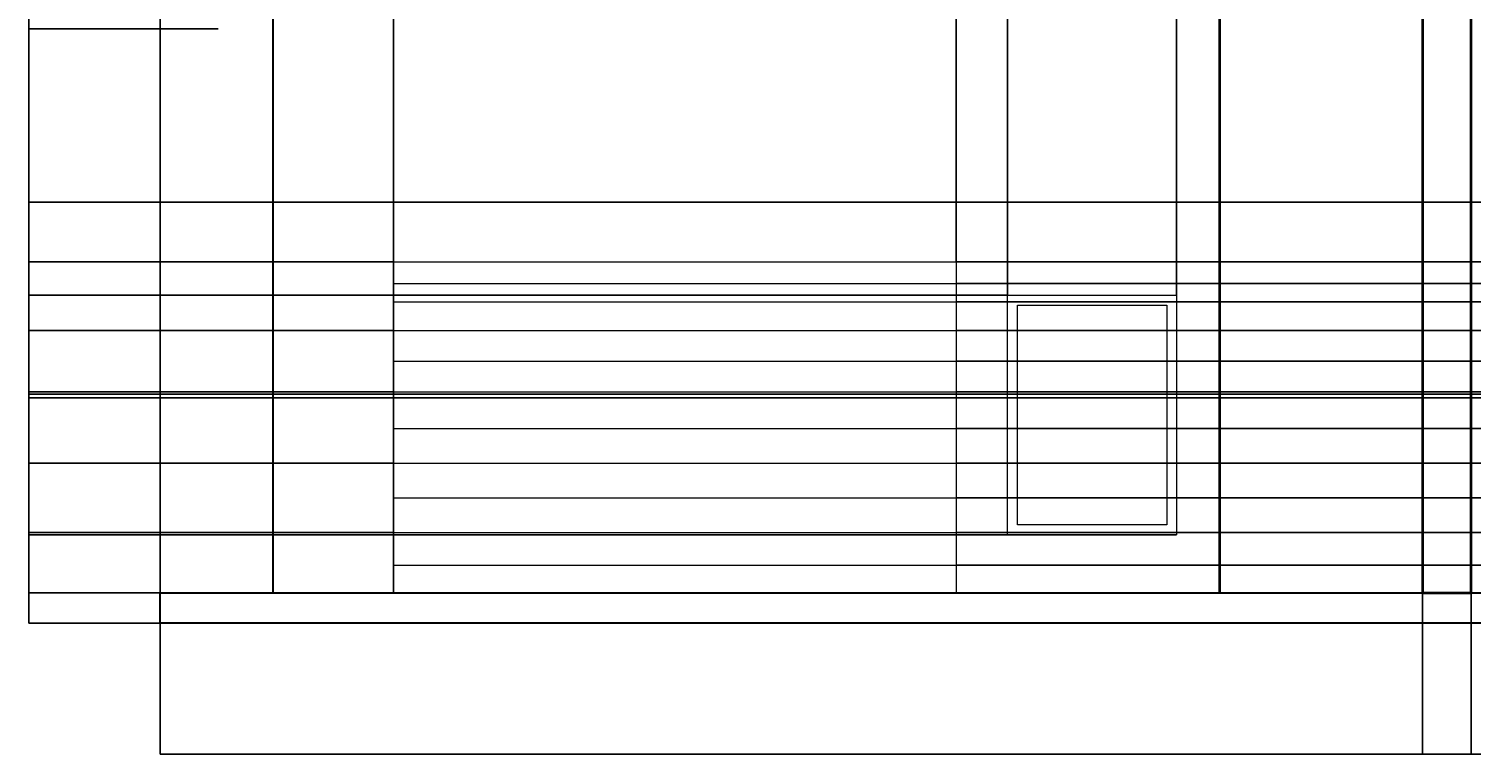
# Model space of a CAD drawing. Units: millimetres. Extents: x 1225 to 9865, y 11 to 4912.
# Tile 1 of 4: x 1225 to 5562, y 11 to 2192. Entities that reach past the tile are written whole.
import ezdxf

# ---------------------------------------------------------------- set-up
doc = ezdxf.new("R2010")
doc.units = ezdxf.units.MM
for name, color, linetype, lineweight in [('A-ANNO-DIMS', 2, 'Continuous', 18), ('A-COLS', 7, 'Continuous', 35), ('A-DOOR', 3, 'Continuous', 20), ('A-GLAZ', 4, 'Continuous', 18), ('A-WALL', 7, 'Continuous', 30), ('S-FNDN', 7, 'Continuous', 30)]:
    doc.layers.add(name, color=color, linetype=linetype, lineweight=lineweight)
doc.styles.get("Standard").update_dxf_attribs({"font": 'arial.ttf'})
doc.dimstyles.get("Standard").update_dxf_attribs({"dimtxt": 0.18, "dimasz": 0.18, "dimexe": 0.18, "dimexo": 0.0625, "dimgap": 0.09, "dimtad": 0, "dimtih": 1, "dimtoh": 1, "dimdec": 4, "dimzin": 0, "dimdsep": 46, "dimtxsty": 'Standard', "dimcen": 0.09, "dimadec": 0, "dimazin": 0, "dimtfac": 1, "dimtdec": 4, "dimtofl": 0, "dimtmove": 0, "dimatfit": 3, "dimfxl": 1, "dimtolj": 1, "dimtzin": 0, "dimarcsym": 0})

# ---------------------------------------------------------------- blocks, each defined once
blk = doc.blocks.new('*D1')
at = {"layer": 'A-ANNO-DIMS', "color": 0, "lineweight": -2, "transparency": 16777216}
for p, q in [((9470.3, 2192.1), (9470.3, 10.6)), ((1619.2, 404.7), (1619.2, 10.6)), ((1619.3, 10.8), (5544.4, 10.8)), ((9470.1, 10.8), (5545.1, 10.8))]:
    blk.add_line(p, q, dxfattribs=at)
at = {"layer": 'A-ANNO-DIMS', "color": 0, "transparency": 16777216}
for points in [[(1619.3, 10.8), (1619.3, 10.7), (1619.2, 10.8)], [(9470.1, 10.8), (9470.1, 10.7), (9470.3, 10.8)]]:
    blk.add_solid(points, dxfattribs=at)
at = {"layer": 'Defpoints', "color": 0, "transparency": 16777216}
for p in [(9470.3, 2192.2), (1619.2, 404.8), (9470.3, 10.8)]:
    blk.add_point(p, dxfattribs=at)
at = {"layer": 'A-ANNO-DIMS', "color": 0, "transparency": 16777216, "insert": (5544.7, 10.8), "char_height": 0.18, "attachment_point": 5}
blk.add_mtext('\\A1;7851', dxfattribs=at)
blk = doc.blocks.new('*D2')
at = {"layer": 'A-ANNO-DIMS', "color": 0, "lineweight": -2, "transparency": 16777216}
for p, q in [((4805.3, 4517.6), (1225, 4517.6)), ((1225.2, 4517.4), (1225.2, 2461.4)), ((1225.2, 404.9), (1225.2, 2461)), ((1619.1, 404.8), (1225, 404.8))]:
    blk.add_line(p, q, dxfattribs=at)
at = {"layer": 'A-ANNO-DIMS', "color": 0, "transparency": 16777216}
for points in [[(1225.1, 4517.4), (1225.2, 4517.4), (1225.2, 4517.6)], [(1225.1, 404.9), (1225.2, 404.9), (1225.2, 404.8)]]:
    blk.add_solid(points, dxfattribs=at)
at = {"layer": 'Defpoints', "color": 0, "transparency": 16777216}
for p in [(1225.2, 4517.6), (4805.4, 4517.6), (1619.2, 404.8)]:
    blk.add_point(p, dxfattribs=at)
at = {"layer": 'A-ANNO-DIMS', "color": 0, "transparency": 16777216, "insert": (1225.2, 2461.2), "char_height": 0.18, "attachment_point": 5}
blk.add_mtext('\\A1;4113', dxfattribs=at)
blk = doc.blocks.new('*D3')
at = {"layer": 'A-ANNO-DIMS', "color": 0, "lineweight": -2, "transparency": 16777216}
for p, q in [((1619.2, 496.3), (1619.2, 4911.8)), ((1619.3, 4911.6), (1789.1, 4911.6)), ((1959.7, 4911.6), (1789.9, 4911.6)), ((1959.9, 496.3), (1959.9, 4911.8))]:
    blk.add_line(p, q, dxfattribs=at)
at = {"layer": 'A-ANNO-DIMS', "color": 0, "transparency": 16777216}
for points in [[(1619.3, 4911.6), (1619.3, 4911.6), (1619.2, 4911.6)], [(1959.7, 4911.6), (1959.7, 4911.6), (1959.9, 4911.6)]]:
    blk.add_solid(points, dxfattribs=at)
at = {"layer": 'Defpoints', "color": 0, "transparency": 16777216}
for p in [(1959.9, 4911.6), (1619.2, 496.3), (1959.9, 496.3)]:
    blk.add_point(p, dxfattribs=at)
at = {"layer": 'A-ANNO-DIMS', "color": 0, "transparency": 16777216, "insert": (1789.5, 4911.6), "char_height": 0.18, "attachment_point": 5}
blk.add_mtext('\\A1;340.7', dxfattribs=at)
blk = doc.blocks.new('*D4')
at = {"layer": 'A-ANNO-DIMS', "color": 0, "lineweight": -2, "transparency": 16777216}
for p, q in [((1959.9, 496.3), (1959.9, 4911.8)), ((1960.1, 4911.6), (2140.3, 4911.6)), ((2321.6, 4911.6), (2141.3, 4911.6)), ((2321.7, 496.3), (2321.7, 4911.8))]:
    blk.add_line(p, q, dxfattribs=at)
at = {"layer": 'A-ANNO-DIMS', "color": 0, "transparency": 16777216}
for points in [[(1960.1, 4911.6), (1960.1, 4911.6), (1959.9, 4911.6)], [(2321.6, 4911.6), (2321.6, 4911.6), (2321.7, 4911.6)]]:
    blk.add_solid(points, dxfattribs=at)
at = {"layer": 'Defpoints', "color": 0, "transparency": 16777216}
for p in [(2321.7, 4911.6), (1959.9, 496.3), (2321.7, 496.3)]:
    blk.add_point(p, dxfattribs=at)
at = {"layer": 'A-ANNO-DIMS', "color": 0, "transparency": 16777216, "insert": (2140.8, 4911.6), "char_height": 0.18, "attachment_point": 5}
blk.add_mtext('\\A1;361.84', dxfattribs=at)
blk = doc.blocks.new('*D5')
at = {"layer": 'A-ANNO-DIMS', "color": 0, "lineweight": -2, "transparency": 16777216}
for p, q in [((2321.7, 1491.6), (2321.7, 4911.8)), ((2321.9, 4911.6), (3167.3, 4911.6)), ((4013.5, 4911.6), (3168, 4911.6)), ((4013.6, 1491.6), (4013.6, 4911.8))]:
    blk.add_line(p, q, dxfattribs=at)
at = {"layer": 'A-ANNO-DIMS', "color": 0, "transparency": 16777216}
for points in [[(2321.9, 4911.6), (2321.9, 4911.6), (2321.7, 4911.6)], [(4013.5, 4911.6), (4013.5, 4911.6), (4013.6, 4911.6)]]:
    blk.add_solid(points, dxfattribs=at)
at = {"layer": 'Defpoints', "color": 0, "transparency": 16777216}
for p in [(4013.6, 4911.6), (2321.7, 1491.5), (4013.6, 1491.5)]:
    blk.add_point(p, dxfattribs=at)
at = {"layer": 'A-ANNO-DIMS', "color": 0, "transparency": 16777216, "insert": (3167.7, 4911.6), "char_height": 0.18, "attachment_point": 5}
blk.add_mtext('\\A1;1692', dxfattribs=at)
blk = doc.blocks.new('*D6')
at = {"layer": 'A-ANNO-DIMS', "color": 0, "lineweight": -2, "transparency": 16777216}
for p, q in [((4013.6, 1491.6), (4013.6, 4911.8)), ((4013.8, 4911.6), (4090.2, 4911.6)), ((4167.3, 4911.6), (4090.9, 4911.6)), ((4167.5, 1391.1), (4167.5, 4911.8))]:
    blk.add_line(p, q, dxfattribs=at)
at = {"layer": 'A-ANNO-DIMS', "color": 0, "transparency": 16777216}
for points in [[(4013.8, 4911.6), (4013.8, 4911.6), (4013.6, 4911.6)], [(4167.3, 4911.6), (4167.3, 4911.6), (4167.5, 4911.6)]]:
    blk.add_solid(points, dxfattribs=at)
at = {"layer": 'Defpoints', "color": 0, "transparency": 16777216}
for p in [(4167.5, 4911.6), (4013.6, 1491.5), (4167.5, 1391.1)]:
    blk.add_point(p, dxfattribs=at)
at = {"layer": 'A-ANNO-DIMS', "color": 0, "transparency": 16777216, "insert": (4090.5, 4911.6), "char_height": 0.18, "attachment_point": 5}
blk.add_mtext('\\A1;153.8', dxfattribs=at)
blk = doc.blocks.new('*D7')
at = {"layer": 'A-ANNO-DIMS', "color": 0, "lineweight": -2, "transparency": 16777216}
for p, q in [((4167.5, 1391.1), (4167.5, 4911.8)), ((4167.6, 4911.6), (4421.4, 4911.6)), ((4676, 4911.6), (4422.2, 4911.6)), ((4676.2, 1391.1), (4676.2, 4911.8))]:
    blk.add_line(p, q, dxfattribs=at)
at = {"layer": 'A-ANNO-DIMS', "color": 0, "transparency": 16777216}
for points in [[(4167.6, 4911.6), (4167.6, 4911.6), (4167.5, 4911.6)], [(4676, 4911.6), (4676, 4911.6), (4676.2, 4911.6)]]:
    blk.add_solid(points, dxfattribs=at)
at = {"layer": 'Defpoints', "color": 0, "transparency": 16777216}
for p in [(4676.2, 4911.6), (4167.5, 1391.1), (4676.2, 1391.1)]:
    blk.add_point(p, dxfattribs=at)
at = {"layer": 'A-ANNO-DIMS', "color": 0, "transparency": 16777216, "insert": (4421.8, 4911.6), "char_height": 0.18, "attachment_point": 5}
blk.add_mtext('\\A1;508.8', dxfattribs=at)
blk = doc.blocks.new('*D9')
at = {"layer": 'A-ANNO-DIMS', "color": 0, "lineweight": -2, "transparency": 16777216}
for p, q in [((5415.4, 4322.4), (5415.4, 10.6)), ((5561.8, 4322.4), (5561.8, 10.6)), ((5415.6, 10.8), (5488.1, 10.8)), ((5561.6, 10.8), (5489, 10.8))]:
    blk.add_line(p, q, dxfattribs=at)
at = {"layer": 'A-ANNO-DIMS', "color": 0, "transparency": 16777216}
for points in [[(5415.6, 10.8), (5415.6, 10.7), (5415.4, 10.8)], [(5561.6, 10.8), (5561.6, 10.7), (5561.8, 10.8)]]:
    blk.add_solid(points, dxfattribs=at)
at = {"layer": 'Defpoints', "color": 0, "transparency": 16777216}
for p in [(5415.4, 4322.4), (5561.8, 4322.4), (5561.8, 10.8)]:
    blk.add_point(p, dxfattribs=at)
at = {"layer": 'A-ANNO-DIMS', "color": 0, "transparency": 16777216, "insert": (5488.6, 10.8), "char_height": 0.18, "attachment_point": 5}
blk.add_mtext('\\A1;146.38', dxfattribs=at)
blk = doc.blocks.new('*D27')
at = {"layer": 'A-ANNO-DIMS', "color": 0, "lineweight": -2, "transparency": 16777216}
for p, q in [((4167.4, 1391.1), (1225, 1391.1)), ((1225.2, 1390.9), (1225.2, 1030.7)), ((1225.2, 670.1), (1225.2, 1030.3)), ((4167.4, 670), (1225, 670))]:
    blk.add_line(p, q, dxfattribs=at)
at = {"layer": 'A-ANNO-DIMS', "color": 0, "transparency": 16777216}
for points in [[(1225.1, 1390.9), (1225.2, 1390.9), (1225.2, 1391.1)], [(1225.1, 670.1), (1225.2, 670.1), (1225.2, 670)]]:
    blk.add_solid(points, dxfattribs=at)
at = {"layer": 'Defpoints', "color": 0, "transparency": 16777216}
for p in [(1225.2, 1391.1), (4167.5, 1391.1), (4167.5, 670)]:
    blk.add_point(p, dxfattribs=at)
at = {"layer": 'A-ANNO-DIMS', "color": 0, "transparency": 16777216, "insert": (1225.2, 1030.5), "char_height": 0.18, "attachment_point": 5}
blk.add_mtext('\\A1;721.1', dxfattribs=at)
blk = doc.blocks.new('*D28')
at = {"layer": 'A-ANNO-DIMS', "color": 0, "lineweight": -2, "transparency": 16777216}
for p, q in [((4676.1, 670), (1225, 670)), ((1225.2, 669.8), (1225.2, 583.3)), ((1225.2, 496.4), (1225.2, 582.9)), ((4805.3, 496.3), (1225, 496.3))]:
    blk.add_line(p, q, dxfattribs=at)
at = {"layer": 'A-ANNO-DIMS', "color": 0, "transparency": 16777216}
for points in [[(1225.1, 669.8), (1225.2, 669.8), (1225.2, 670)], [(1225.1, 496.4), (1225.2, 496.4), (1225.2, 496.3)]]:
    blk.add_solid(points, dxfattribs=at)
at = {"layer": 'Defpoints', "color": 0, "transparency": 16777216}
for p in [(4676.2, 670), (1225.2, 496.3), (4805.4, 496.3)]:
    blk.add_point(p, dxfattribs=at)
at = {"layer": 'A-ANNO-DIMS', "color": 0, "transparency": 16777216, "insert": (1225.2, 583.1), "char_height": 0.18, "attachment_point": 5}
blk.add_mtext('\\A1;173.7', dxfattribs=at)
blk = doc.blocks.new('*D29')
at = {"layer": 'A-ANNO-DIMS', "color": 0, "lineweight": -2, "transparency": 16777216}
for p, q in [((1794.1, 2192.2), (1225, 2192.2)), ((1225.2, 2192), (1225.2, 1344.4)), ((1225.2, 496.4), (1225.2, 1344)), ((1959.8, 496.3), (1225, 496.3))]:
    blk.add_line(p, q, dxfattribs=at)
at = {"layer": 'A-ANNO-DIMS', "color": 0, "transparency": 16777216}
for points in [[(1225.1, 2192), (1225.2, 2192), (1225.2, 2192.2)], [(1225.1, 496.4), (1225.2, 496.4), (1225.2, 496.3)]]:
    blk.add_solid(points, dxfattribs=at)
at = {"layer": 'Defpoints', "color": 0, "transparency": 16777216}
for p in [(1225.2, 2192.2), (1794.2, 2192.2), (1959.9, 496.3)]:
    blk.add_point(p, dxfattribs=at)
at = {"layer": 'A-ANNO-DIMS', "color": 0, "transparency": 16777216, "insert": (1225.2, 1344.2), "char_height": 0.18, "attachment_point": 5}
blk.add_mtext('\\A1;1696', dxfattribs=at)
blk = doc.blocks.new('*D38')
at = {"layer": 'A-ANNO-DIMS', "color": 0, "lineweight": -2, "transparency": 16777216}
for p, q in [((6393, 1670.8), (1225, 1670.8)), ((1225.2, 1670.7), (1225.2, 1083.7)), ((1225.2, 496.4), (1225.2, 1083.4)), ((6393, 496.3), (1225, 496.3))]:
    blk.add_line(p, q, dxfattribs=at)
at = {"layer": 'A-ANNO-DIMS', "color": 0, "transparency": 16777216}
for points in [[(1225.1, 1670.7), (1225.2, 1670.7), (1225.2, 1670.8)], [(1225.1, 496.4), (1225.2, 496.4), (1225.2, 496.3)]]:
    blk.add_solid(points, dxfattribs=at)
at = {"layer": 'Defpoints', "color": 0, "transparency": 16777216}
for p in [(1225.2, 1670.8), (6393.1, 1670.8), (6393.1, 496.3)]:
    blk.add_point(p, dxfattribs=at)
at = {"layer": 'A-ANNO-DIMS', "color": 0, "transparency": 16777216, "insert": (1225.2, 1083.6), "char_height": 0.18, "attachment_point": 5}
blk.add_mtext('\\A1;1174.6', dxfattribs=at)
blk = doc.blocks.new('*D39')
at = {"layer": 'A-ANNO-DIMS', "color": 0, "lineweight": -2, "transparency": 16777216}
for p, q in [((7484.2, 1670.8), (1225, 1670.8)), ((1225.2, 1670.7), (1225.2, 1382.4)), ((1225.2, 1093.8), (1225.2, 1382.1)), ((7484.2, 1093.7), (1225, 1093.7))]:
    blk.add_line(p, q, dxfattribs=at)
at = {"layer": 'A-ANNO-DIMS', "color": 0, "transparency": 16777216}
for points in [[(1225.1, 1670.7), (1225.2, 1670.7), (1225.2, 1670.8)], [(1225.1, 1093.8), (1225.2, 1093.8), (1225.2, 1093.7)]]:
    blk.add_solid(points, dxfattribs=at)
at = {"layer": 'Defpoints', "color": 0, "transparency": 16777216}
for p in [(1225.2, 1670.8), (7484.2, 1670.8), (7484.2, 1093.7)]:
    blk.add_point(p, dxfattribs=at)
at = {"layer": 'A-ANNO-DIMS', "color": 0, "transparency": 16777216, "insert": (1225.2, 1382.3), "char_height": 0.18, "attachment_point": 5}
blk.add_mtext('\\A1;577.2', dxfattribs=at)
blk = doc.blocks.new('*D44')
at = {"layer": 'A-ANNO-DIMS', "color": 0, "lineweight": -2, "transparency": 16777216}
for p, q in [((6983.8, 1081.9), (1225, 1081.9)), ((1225.2, 1081.8), (1225.2, 789.3)), ((1225.2, 496.4), (1225.2, 788.9)), ((7138.8, 496.3), (1225, 496.3))]:
    blk.add_line(p, q, dxfattribs=at)
at = {"layer": 'A-ANNO-DIMS', "color": 0, "transparency": 16777216}
for points in [[(1225.1, 1081.8), (1225.2, 1081.8), (1225.2, 1081.9)], [(1225.1, 496.4), (1225.2, 496.4), (1225.2, 496.3)]]:
    blk.add_solid(points, dxfattribs=at)
at = {"layer": 'Defpoints', "color": 0, "transparency": 16777216}
for p in [(6983.8, 1081.9), (1225.2, 496.3), (7138.8, 496.3)]:
    blk.add_point(p, dxfattribs=at)
at = {"layer": 'A-ANNO-DIMS', "color": 0, "transparency": 16777216, "insert": (1225.2, 789.1), "char_height": 0.18, "attachment_point": 5}
blk.add_mtext('\\A1;585.7', dxfattribs=at)
blk = doc.blocks.new('*D62')
at = {"layer": 'A-ANNO-DIMS', "color": 0, "lineweight": -2, "transparency": 16777216}
for p, q in [((2321.7, 677.4), (1225, 677.4)), ((1225.2, 677.2), (1225.2, 587)), ((1225.2, 496.4), (1225.2, 586.6)), ((2321.7, 496.3), (1225, 496.3))]:
    blk.add_line(p, q, dxfattribs=at)
at = {"layer": 'A-ANNO-DIMS', "color": 0, "transparency": 16777216}
for points in [[(1225.1, 677.2), (1225.2, 677.2), (1225.2, 677.4)], [(1225.1, 496.4), (1225.2, 496.4), (1225.2, 496.3)]]:
    blk.add_solid(points, dxfattribs=at)
at = {"layer": 'Defpoints', "color": 0, "transparency": 16777216}
for p in [(1225.2, 677.4), (2321.7, 677.4), (2321.7, 496.3)]:
    blk.add_point(p, dxfattribs=at)
at = {"layer": 'A-ANNO-DIMS', "color": 0, "transparency": 16777216, "insert": (1225.2, 586.8), "char_height": 0.18, "attachment_point": 5}
blk.add_mtext('\\A1;181.13', dxfattribs=at)
blk = doc.blocks.new('*D63')
at = {"layer": 'A-ANNO-DIMS', "color": 0, "lineweight": -2, "transparency": 16777216}
for p, q in [((2321.7, 886), (1225, 886)), ((1225.2, 885.8), (1225.2, 781.9)), ((1225.2, 677.6), (1225.2, 781.5)), ((2321.7, 677.4), (1225, 677.4))]:
    blk.add_line(p, q, dxfattribs=at)
at = {"layer": 'A-ANNO-DIMS', "color": 0, "transparency": 16777216}
for points in [[(1225.1, 885.8), (1225.2, 885.8), (1225.2, 886)], [(1225.1, 677.6), (1225.2, 677.6), (1225.2, 677.4)]]:
    blk.add_solid(points, dxfattribs=at)
at = {"layer": 'Defpoints', "color": 0, "transparency": 16777216}
for p in [(1225.2, 886), (2321.7, 886), (2321.7, 677.4)]:
    blk.add_point(p, dxfattribs=at)
at = {"layer": 'A-ANNO-DIMS', "color": 0, "transparency": 16777216, "insert": (1225.2, 781.7), "char_height": 0.18, "attachment_point": 5}
blk.add_mtext('\\A1;208.6', dxfattribs=at)
blk = doc.blocks.new('*D64')
at = {"layer": 'A-ANNO-DIMS', "color": 0, "lineweight": -2, "transparency": 16777216}
for p, q in [((2321.7, 1100.8), (1225, 1100.8)), ((1225.2, 1100.6), (1225.2, 993.6)), ((1225.2, 886.2), (1225.2, 993.2)), ((2321.7, 886), (1225, 886))]:
    blk.add_line(p, q, dxfattribs=at)
at = {"layer": 'A-ANNO-DIMS', "color": 0, "transparency": 16777216}
for points in [[(1225.1, 1100.6), (1225.2, 1100.6), (1225.2, 1100.8)], [(1225.1, 886.2), (1225.2, 886.2), (1225.2, 886)]]:
    blk.add_solid(points, dxfattribs=at)
at = {"layer": 'Defpoints', "color": 0, "transparency": 16777216}
for p in [(1225.2, 1100.8), (2321.7, 1100.8), (2321.7, 886)]:
    blk.add_point(p, dxfattribs=at)
at = {"layer": 'A-ANNO-DIMS', "color": 0, "transparency": 16777216, "insert": (1225.2, 993.4), "char_height": 0.18, "attachment_point": 5}
blk.add_mtext('\\A1;214.75', dxfattribs=at)
blk = doc.blocks.new('*D65')
at = {"layer": 'A-ANNO-DIMS', "color": 0, "lineweight": -2, "transparency": 16777216}
for p, q in [((2321.7, 1284.8), (1225, 1284.8)), ((1225.2, 1284.7), (1225.2, 1193)), ((1225.2, 1100.9), (1225.2, 1192.6)), ((2321.7, 1100.8), (1225, 1100.8))]:
    blk.add_line(p, q, dxfattribs=at)
at = {"layer": 'A-ANNO-DIMS', "color": 0, "transparency": 16777216}
for points in [[(1225.1, 1284.7), (1225.2, 1284.7), (1225.2, 1284.8)], [(1225.1, 1100.9), (1225.2, 1100.9), (1225.2, 1100.8)]]:
    blk.add_solid(points, dxfattribs=at)
at = {"layer": 'Defpoints', "color": 0, "transparency": 16777216}
for p in [(1225.2, 1284.8), (2321.7, 1284.8), (2321.7, 1100.8)]:
    blk.add_point(p, dxfattribs=at)
at = {"layer": 'A-ANNO-DIMS', "color": 0, "transparency": 16777216, "insert": (1225.2, 1192.8), "char_height": 0.18, "attachment_point": 5}
blk.add_mtext('\\A1;184.07', dxfattribs=at)
blk = doc.blocks.new('*D66')
at = {"layer": 'A-ANNO-DIMS', "color": 0, "lineweight": -2, "transparency": 16777216}
for p, q in [((2321.7, 1491.5), (1225, 1491.5)), ((1225.2, 1491.4), (1225.2, 1388.4)), ((1225.2, 1285), (1225.2, 1388)), ((2321.7, 1284.8), (1225, 1284.8))]:
    blk.add_line(p, q, dxfattribs=at)
at = {"layer": 'A-ANNO-DIMS', "color": 0, "transparency": 16777216}
for points in [[(1225.1, 1491.4), (1225.2, 1491.4), (1225.2, 1491.5)], [(1225.1, 1285), (1225.2, 1285), (1225.2, 1284.8)]]:
    blk.add_solid(points, dxfattribs=at)
at = {"layer": 'Defpoints', "color": 0, "transparency": 16777216}
for p in [(1225.2, 1491.5), (2321.7, 1491.5), (2321.7, 1284.8)]:
    blk.add_point(p, dxfattribs=at)
at = {"layer": 'A-ANNO-DIMS', "color": 0, "transparency": 16777216, "insert": (1225.2, 1388.2), "char_height": 0.18, "attachment_point": 5}
blk.add_mtext('\\A1;206.7', dxfattribs=at)
blk = doc.blocks.new('*D67')
at = {"layer": 'A-ANNO-DIMS', "color": 0, "lineweight": -2, "transparency": 16777216}
for p, q in [((4013.7, 579.2), (9864.4, 579.2)), ((9864.3, 579), (9864.3, 537.9)), ((9864.3, 496.4), (9864.3, 537.6)), ((4013.7, 496.3), (9864.4, 496.3))]:
    blk.add_line(p, q, dxfattribs=at)
at = {"layer": 'A-ANNO-DIMS', "color": 0, "transparency": 16777216}
for points in [[(9864.2, 579), (9864.3, 579), (9864.3, 579.2)], [(9864.2, 496.4), (9864.3, 496.4), (9864.3, 496.3)]]:
    blk.add_solid(points, dxfattribs=at)
at = {"layer": 'Defpoints', "color": 0, "transparency": 16777216}
for p in [(4013.6, 579.2), (9864.3, 579.2), (4013.6, 496.3)]:
    blk.add_point(p, dxfattribs=at)
at = {"layer": 'A-ANNO-DIMS', "color": 0, "transparency": 16777216, "insert": (9864.3, 537.7), "char_height": 0.18, "attachment_point": 5}
blk.add_mtext('\\A1;82.96', dxfattribs=at)
blk = doc.blocks.new('*D68')
at = {"layer": 'A-ANNO-DIMS', "color": 0, "lineweight": -2, "transparency": 16777216}
for p, q in [((4013.7, 781.7), (9864.4, 781.7)), ((9864.3, 781.5), (9864.3, 729.7)), ((9864.3, 677.6), (9864.3, 729.4)), ((4013.7, 677.4), (9864.4, 677.4))]:
    blk.add_line(p, q, dxfattribs=at)
at = {"layer": 'A-ANNO-DIMS', "color": 0, "transparency": 16777216}
for points in [[(9864.2, 781.5), (9864.3, 781.5), (9864.3, 781.7)], [(9864.2, 677.6), (9864.3, 677.6), (9864.3, 677.4)]]:
    blk.add_solid(points, dxfattribs=at)
at = {"layer": 'Defpoints', "color": 0, "transparency": 16777216}
for p in [(4013.6, 781.7), (9864.3, 781.7), (4013.6, 677.4)]:
    blk.add_point(p, dxfattribs=at)
at = {"layer": 'A-ANNO-DIMS', "color": 0, "transparency": 16777216, "insert": (9864.3, 729.5), "char_height": 0.18, "attachment_point": 5}
blk.add_mtext('\\A1;104.3', dxfattribs=at)
blk = doc.blocks.new('*D69')
at = {"layer": 'A-ANNO-DIMS', "color": 0, "lineweight": -2, "transparency": 16777216}
for p, q in [((4013.7, 990.3), (9864.4, 990.3)), ((9864.3, 990.1), (9864.3, 938.3)), ((9864.3, 886.2), (9864.3, 938)), ((4013.7, 886), (9864.4, 886))]:
    blk.add_line(p, q, dxfattribs=at)
at = {"layer": 'A-ANNO-DIMS', "color": 0, "transparency": 16777216}
for points in [[(9864.2, 990.1), (9864.3, 990.1), (9864.3, 990.3)], [(9864.2, 886.2), (9864.3, 886.2), (9864.3, 886)]]:
    blk.add_solid(points, dxfattribs=at)
at = {"layer": 'Defpoints', "color": 0, "transparency": 16777216}
for p in [(4013.6, 990.3), (9864.3, 990.3), (4013.6, 886)]:
    blk.add_point(p, dxfattribs=at)
at = {"layer": 'A-ANNO-DIMS', "color": 0, "transparency": 16777216, "insert": (9864.3, 938.2), "char_height": 0.18, "attachment_point": 5}
blk.add_mtext('\\A1;104.3', dxfattribs=at)
blk = doc.blocks.new('*D70')
at = {"layer": 'A-ANNO-DIMS', "color": 0, "lineweight": -2, "transparency": 16777216}
for p, q in [((4013.7, 1192.8), (9864.4, 1192.8)), ((9864.3, 1192.6), (9864.3, 1147)), ((9864.3, 1100.9), (9864.3, 1146.6)), ((4013.7, 1100.8), (9864.4, 1100.8))]:
    blk.add_line(p, q, dxfattribs=at)
at = {"layer": 'A-ANNO-DIMS', "color": 0, "transparency": 16777216}
for points in [[(9864.2, 1192.6), (9864.3, 1192.6), (9864.3, 1192.8)], [(9864.2, 1100.9), (9864.3, 1100.9), (9864.3, 1100.8)]]:
    blk.add_solid(points, dxfattribs=at)
at = {"layer": 'Defpoints', "color": 0, "transparency": 16777216}
for p in [(4013.6, 1192.8), (9864.3, 1192.8), (4013.6, 1100.8)]:
    blk.add_point(p, dxfattribs=at)
at = {"layer": 'A-ANNO-DIMS', "color": 0, "transparency": 16777216, "insert": (9864.3, 1146.8), "char_height": 0.18, "attachment_point": 5}
blk.add_mtext('\\A1;92.04', dxfattribs=at)
blk = doc.blocks.new('*D71')
at = {"layer": 'A-ANNO-DIMS', "color": 0, "lineweight": -2, "transparency": 16777216}
for p, q in [((4013.7, 1370.7), (9864.4, 1370.7)), ((9864.3, 1370.6), (9864.3, 1328)), ((9864.3, 1285), (9864.3, 1327.6)), ((4013.7, 1284.8), (9864.4, 1284.8))]:
    blk.add_line(p, q, dxfattribs=at)
at = {"layer": 'A-ANNO-DIMS', "color": 0, "transparency": 16777216}
for points in [[(9864.2, 1370.6), (9864.3, 1370.6), (9864.3, 1370.7)], [(9864.2, 1285), (9864.3, 1285), (9864.3, 1284.8)]]:
    blk.add_solid(points, dxfattribs=at)
at = {"layer": 'Defpoints', "color": 0, "transparency": 16777216}
for p in [(4013.6, 1370.7), (9864.3, 1370.7), (4013.6, 1284.8)]:
    blk.add_point(p, dxfattribs=at)
at = {"layer": 'A-ANNO-DIMS', "color": 0, "transparency": 16777216, "insert": (9864.3, 1327.8), "char_height": 0.18, "attachment_point": 5}
blk.add_mtext('\\A1;85.9', dxfattribs=at)
blk = doc.blocks.new('*D72')
at = {"layer": 'A-ANNO-DIMS', "color": 0, "lineweight": -2, "transparency": 16777216}
for p, q in [((4013.7, 1491.5), (9864.4, 1491.5)), ((9864.3, 1491.4), (9864.3, 1459.1)), ((9864.3, 1426.6), (9864.3, 1458.8)), ((4013.7, 1426.4), (9864.4, 1426.4))]:
    blk.add_line(p, q, dxfattribs=at)
at = {"layer": 'A-ANNO-DIMS', "color": 0, "transparency": 16777216}
for points in [[(9864.2, 1491.4), (9864.3, 1491.4), (9864.3, 1491.5)], [(9864.2, 1426.6), (9864.3, 1426.6), (9864.3, 1426.4)]]:
    blk.add_solid(points, dxfattribs=at)
at = {"layer": 'Defpoints', "color": 0, "transparency": 16777216}
for p in [(4013.6, 1491.5), (9864.3, 1491.5), (4013.6, 1426.4)]:
    blk.add_point(p, dxfattribs=at)
at = {"layer": 'A-ANNO-DIMS', "color": 0, "transparency": 16777216, "insert": (9864.3, 1459), "char_height": 0.18, "attachment_point": 5}
blk.add_mtext('\\A1;65.16', dxfattribs=at)

msp = doc.modelspace()

# ---------------------------------------------------------------- linework, layer by layer
at = {"layer": 'A-COLS'}
for p, q in [((5415.376, 4517.596), (5415.376, 496.264)), ((5561.752, 496.264), (5561.752, 4517.596)), ((4805.396, 3949.397), (4805.396, 496.264)), ((5415.376, 496.264), (5561.752, 496.264))]:
    msp.add_line(p, q, dxfattribs=at)
at = {"layer": 'A-DOOR'}
for p, q in [((2321.73, 496.264), (2321.73, 1491.543)), ((2321.73, 1491.543), (4013.642, 1491.543)), ((4013.642, 1491.543), (4013.642, 496.264)), ((2321.73, 1426.384), (4013.642, 1426.384)), ((2321.73, 1370.736), (4013.642, 1370.736)), ((2321.73, 1284.835), (4013.642, 1284.835)), ((2321.73, 1192.799), (4013.642, 1192.799)), ((2321.73, 1100.763), (4013.642, 1100.763)), ((2321.73, 990.319), (4013.642, 990.319)), ((2321.73, 886.011), (4013.642, 886.011)), ((2321.73, 781.703), (4013.642, 781.703)), ((2321.73, 677.396), (4013.642, 677.396)), ((2321.73, 579.223), (4013.642, 579.223))]:
    msp.add_line(p, q, dxfattribs=at)
at = {"layer": 'A-GLAZ'}
for points in [[(4167.452, 1391.062), (4676.209, 1391.062), (4676.209, 669.957), (4167.452, 669.957)], [(4197.452, 1361.062), (4646.209, 1361.062), (4646.209, 699.957), (4197.452, 699.957)]]:
    msp.add_lwpolyline(points, close=True, dxfattribs=at)
at = {"layer": 'A-WALL'}
msp.add_line((1959.893, 496.264), (1959.893, 3949.397), dxfattribs=at)
at = {"layer": 'S-FNDN'}
for p, q in [((1619.167, 496.264), (6462.269, 496.264)), ((1619.167, 404.75), (1619.167, 496.264)), ((6462.269, 404.75), (1619.167, 404.75))]:
    msp.add_line(p, q, dxfattribs=at)

# ---------------------------------------------------------------- dimensions: what is measured, and where the dimension line sits
at = {"layer": 'A-ANNO-DIMS'}
for base, p1, p2, override, picture, middle in [((1959.893, 4911.596), (1619.167, 496.264), (1959.893, 496.264), {"dimdec": 1, "dimlfac": 1, "dimrnd": 0, "dimzin": 0, "dimdsep": 46, "dimlunit": 2}, '*D3', (1789.53, 4911.596)), ((2321.73, 4911.596), (1959.893, 496.264), (2321.73, 496.264), {"dimdec": 2, "dimlfac": 1, "dimrnd": 0, "dimzin": 0, "dimdsep": 46, "dimlunit": 2}, '*D4', (2140.812, 4911.596)), ((4013.642, 4911.596), (2321.73, 1491.543), (4013.642, 1491.543), {"dimdec": 0, "dimlfac": 1, "dimrnd": 0, "dimzin": 0, "dimdsep": 46, "dimlunit": 2}, '*D5', (3167.686, 4911.596)), ((4167.452, 4911.596), (4013.642, 1491.543), (4167.452, 1391.062), {"dimdec": 1, "dimlfac": 1, "dimrnd": 0, "dimzin": 0, "dimdsep": 46, "dimlunit": 2}, '*D6', (4090.547, 4911.596)), ((4676.209, 4911.596), (4167.452, 1391.062), (4676.209, 1391.062), {"dimdec": 1, "dimlfac": 1, "dimrnd": 0, "dimzin": 0, "dimdsep": 46, "dimlunit": 2}, '*D7', (4421.831, 4911.596)), ((5561.752, 10.75), (5415.376, 4322.413), (5561.752, 4322.413), {"dimdec": 2, "dimlfac": 1, "dimrnd": 0, "dimzin": 0, "dimdsep": 46, "dimlunit": 2}, '*D9', (5488.564, 10.75)), ((9470.268, 10.75), (1619.167, 404.75), (9470.268, 2192.169), {"dimdec": 0, "dimlfac": 1, "dimrnd": 0, "dimzin": 0, "dimdsep": 46, "dimlunit": 2}, '*D1', (5544.717, 10.75))]:
    dim = msp.add_linear_dim(base=base, p1=p1, p2=p2, dimstyle='Standard', override=override, dxfattribs=at)
    dim.commit()
    dim.dimension.update_dxf_attribs({"geometry": picture, "text_midpoint": middle})
for base, p1, p2, override, picture, middle in [((1225.167, 4517.596), (1619.167, 404.75), (4805.396, 4517.596), {"dimdec": 0, "dimlfac": 1, "dimrnd": 0, "dimzin": 0, "dimdsep": 46, "dimlunit": 2}, '*D2', (1225.167, 2461.173)), ((1225.167, 2192.169), (1959.893, 496.264), (1794.21, 2192.169), {"dimdec": 0, "dimlfac": 1, "dimrnd": 0, "dimzin": 0, "dimdsep": 46, "dimlunit": 2}, '*D29', (1225.167, 1344.216)), ((1225.167, 1670.836), (6393.055, 496.264), (6393.055, 1670.836), {"dimdec": 1, "dimlfac": 1, "dimrnd": 0, "dimzin": 0, "dimdsep": 46, "dimlunit": 2}, '*D38', (1225.167, 1083.55)), ((1225.167, 1670.836), (7484.241, 1093.666), (7484.241, 1670.836), {"dimdec": 1, "dimlfac": 1, "dimrnd": 0, "dimzin": 0, "dimdsep": 46, "dimlunit": 2}, '*D39', (1225.167, 1382.251)), ((1225.167, 1491.543), (2321.73, 1284.835), (2321.73, 1491.543), {"dimdec": 1, "dimlfac": 1, "dimrnd": 0, "dimzin": 0, "dimdsep": 46, "dimlunit": 2}, '*D66', (1225.167, 1388.189)), ((9864.268, 1491.543), (4013.642, 1426.384), (4013.642, 1491.543), {"dimdec": 2, "dimlfac": 1, "dimrnd": 0, "dimzin": 0, "dimdsep": 46, "dimlunit": 2}, '*D72', (9864.268, 1458.964)), ((1225.167, 1391.062), (4167.452, 669.957), (4167.452, 1391.062), {"dimdec": 1, "dimlfac": 1, "dimrnd": 0, "dimzin": 0, "dimdsep": 46, "dimlunit": 2}, '*D27', (1225.167, 1030.51)), ((9864.268, 1370.736), (4013.642, 1284.835), (4013.642, 1370.736), {"dimdec": 1, "dimlfac": 1, "dimrnd": 0, "dimzin": 0, "dimdsep": 46, "dimlunit": 2}, '*D71', (9864.268, 1327.786)), ((1225.167, 1284.835), (2321.73, 1100.763), (2321.73, 1284.835), {"dimdec": 2, "dimlfac": 1, "dimrnd": 0, "dimzin": 0, "dimdsep": 46, "dimlunit": 2}, '*D65', (1225.167, 1192.799)), ((9864.268, 1192.799), (4013.642, 1100.763), (4013.642, 1192.799), {"dimdec": 2, "dimlfac": 1, "dimrnd": 0, "dimzin": 0, "dimdsep": 46, "dimlunit": 2}, '*D70', (9864.268, 1146.781)), ((1225.167, 1100.763), (2321.73, 886.011), (2321.73, 1100.763), {"dimdec": 2, "dimlfac": 1, "dimrnd": 0, "dimzin": 0, "dimdsep": 46, "dimlunit": 2}, '*D64', (1225.167, 993.387)), ((1225.167, 496.264), (6983.847, 1081.944), (7138.844, 496.264), {"dimdec": 1, "dimlfac": 1, "dimrnd": 0, "dimzin": 0, "dimdsep": 46, "dimlunit": 2}, '*D44', (1225.167, 789.104)), ((9864.268, 990.319), (4013.642, 886.011), (4013.642, 990.319), {"dimdec": 1, "dimlfac": 1, "dimrnd": 0, "dimzin": 0, "dimdsep": 46, "dimlunit": 2}, '*D69', (9864.268, 938.165)), ((1225.167, 886.011), (2321.73, 677.396), (2321.73, 886.011), {"dimdec": 1, "dimlfac": 1, "dimrnd": 0, "dimzin": 0, "dimdsep": 46, "dimlunit": 2}, '*D63', (1225.167, 781.703)), ((9864.268, 781.703), (4013.642, 677.396), (4013.642, 781.703), {"dimdec": 1, "dimlfac": 1, "dimrnd": 0, "dimzin": 0, "dimdsep": 46, "dimlunit": 2}, '*D68', (9864.268, 729.549)), ((1225.167, 677.396), (2321.73, 496.264), (2321.73, 677.396), {"dimdec": 2, "dimlfac": 1, "dimrnd": 0, "dimzin": 0, "dimdsep": 46, "dimlunit": 2}, '*D62', (1225.167, 586.83)), ((1225.167, 496.264), (4676.209, 669.957), (4805.396, 496.264), {"dimdec": 1, "dimlfac": 1, "dimrnd": 0, "dimzin": 0, "dimdsep": 46, "dimlunit": 2}, '*D28', (1225.167, 583.111)), ((9864.268, 579.223), (4013.642, 496.264), (4013.642, 579.223), {"dimdec": 2, "dimlfac": 1, "dimrnd": 0, "dimzin": 0, "dimdsep": 46, "dimlunit": 2}, '*D67', (9864.268, 537.744))]:
    dim = msp.add_linear_dim(base=base, p1=p1, p2=p2, angle=90, dimstyle='Standard', override=override, dxfattribs=at)
    dim.commit()
    dim.dimension.update_dxf_attribs({"geometry": picture, "text_midpoint": middle})

doc.saveas('drawing.dxf')
